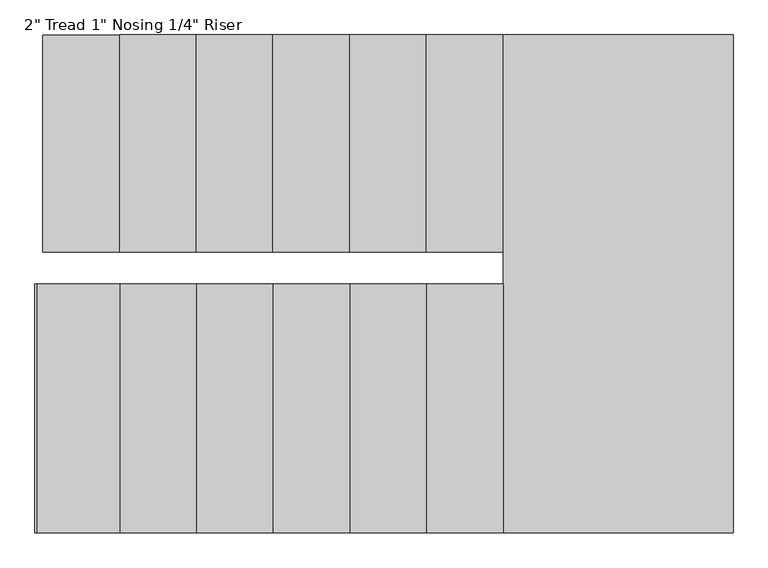
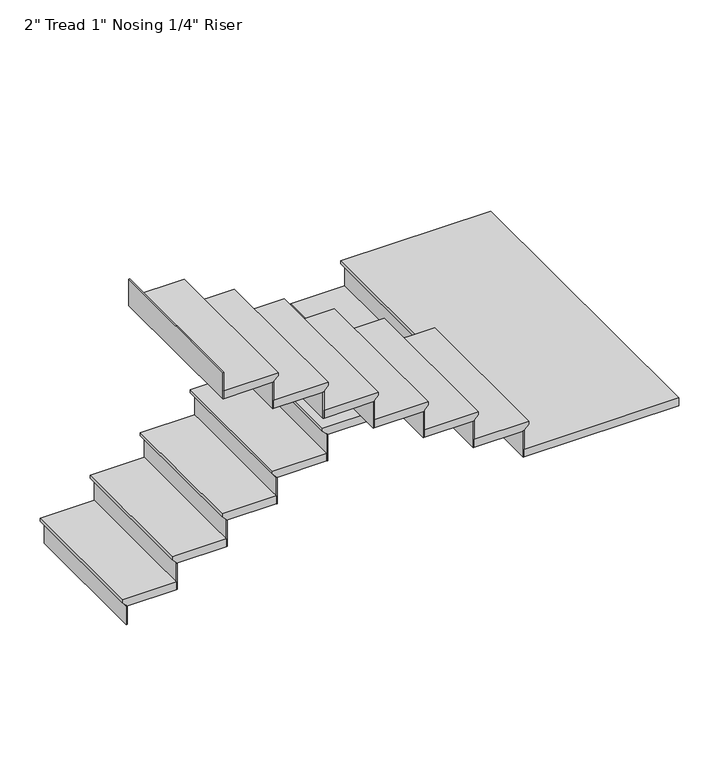
"""IFC4 building model written with IfcOpenShell, lengths in millimetres: stair flight geometry."""

from ifc_helpers import new_model, si_unit, origin, place, context, project, spatial, faceted_brep, source, transform, mapped, element, save


def stair_flight_2c0e0b85(model_context):
    return source(origin(), model_context, "Body", "Brep", [
        faceted_brep([(-879.540747, -2928.9064015, 150.2833333), (-879.540747, -2928.9064015, 169.3333333), (-879.540747, -2065.3064015, 169.3333333), (-879.540747, -2065.3064015, 150.2833333), (-854.140747, -2928.9064015, 124.8833333), (-854.140747, -2065.3064015, 124.8833333), (-549.340747, -2928.9064015, 169.3333333), (-549.340747, -2065.3064015, 169.3333333), (-854.140747, -2065.3064015, 118.5333333), (-549.340747, -2065.3064015, 118.5333333), (-549.340747, -2928.9064015, 118.5333333), (-854.140747, -2928.9064015, 118.5333333)], [[[0, 1, 2, 3]], [[4, 0, 3, 5]], [[2, 1, 6, 7]], [[8, 9, 10, 11]], [[2, 7, 9, 8, 5, 3]], [[8, 11, 4, 5]], [[6, 1, 0, 4, 11, 10]], [[7, 6, 10, 9]]]),
        faceted_brep([(-854.140747, -2928.9064015, 118.5333333), (-854.140747, -2928.9064015, 0.0), (-847.790747, -2928.9064015, 0.0), (-847.790747, -2928.9064015, 118.5333333), (-854.140747, -2065.3064015, 118.5333333), (-847.790747, -2065.3064015, 118.5333333), (-847.790747, -2065.3064015, 0.0), (-854.140747, -2065.3064015, 0.0)], [[[0, 1, 2, 3]], [[4, 5, 6, 7]], [[1, 0, 4, 7]], [[2, 1, 7, 6]], [[3, 2, 6, 5]], [[0, 3, 5, 4]]]),
        faceted_brep([(-549.340747, -2928.9064015, 287.8666667), (-549.340747, -2928.9064015, 118.5333333), (-542.990747, -2928.9064015, 118.5333333), (-542.990747, -2928.9064015, 287.8666667), (-549.340747, -2065.3064015, 287.8666667), (-542.990747, -2065.3064015, 287.8666667), (-542.990747, -2065.3064015, 118.5333333), (-549.340747, -2065.3064015, 118.5333333)], [[[0, 1, 2, 3]], [[4, 5, 6, 7]], [[1, 0, 4, 7]], [[2, 1, 7, 6]], [[3, 2, 6, 5]], [[0, 3, 5, 4]]]),
        faceted_brep([(-574.740747, -2065.3064015, 338.6666667), (-574.740747, -2928.9064015, 338.6666667), (-244.540747, -2928.9064015, 338.6666667), (-244.540747, -2065.3064015, 338.6666667), (-549.340747, -2065.3064015, 287.8666667), (-244.540747, -2065.3064015, 287.8666667), (-244.540747, -2928.9064015, 287.8666667), (-549.340747, -2928.9064015, 287.8666667), (-549.340747, -2065.3064015, 294.2166667), (-574.740747, -2065.3064015, 319.6166667), (-549.340747, -2928.9064015, 294.2166667), (-574.740747, -2928.9064015, 319.6166667)], [[[0, 1, 2, 3]], [[4, 5, 6, 7]], [[0, 3, 5, 4, 8, 9]], [[4, 7, 10, 8]], [[2, 1, 11, 10, 7, 6]], [[3, 2, 6, 5]], [[11, 1, 0, 9]], [[10, 11, 9, 8]]]),
        faceted_brep([(-244.540747, -2928.9064015, 457.2), (-244.540747, -2928.9064015, 287.8666667), (-238.190747, -2928.9064015, 287.8666667), (-238.190747, -2928.9064015, 457.2), (-244.540747, -2065.3064015, 457.2), (-238.190747, -2065.3064015, 457.2), (-238.190747, -2065.3064015, 287.8666667), (-244.540747, -2065.3064015, 287.8666667)], [[[0, 1, 2, 3]], [[4, 5, 6, 7]], [[1, 0, 4, 7]], [[2, 1, 7, 6]], [[3, 2, 6, 5]], [[0, 3, 5, 4]]]),
        faceted_brep([(-269.940747, -2065.3064015, 508.0), (-269.940747, -2928.9064015, 508.0), (60.259253, -2928.9064015, 508.0), (60.259253, -2065.3064015, 508.0), (-244.540747, -2065.3064015, 457.2), (60.259253, -2065.3064015, 457.2), (60.259253, -2928.9064015, 457.2), (-244.540747, -2928.9064015, 457.2), (-244.540747, -2065.3064015, 463.55), (-269.940747, -2065.3064015, 488.95), (-244.540747, -2928.9064015, 463.55), (-269.940747, -2928.9064015, 488.95)], [[[0, 1, 2, 3]], [[4, 5, 6, 7]], [[0, 3, 5, 4, 8, 9]], [[4, 7, 10, 8]], [[2, 1, 11, 10, 7, 6]], [[3, 2, 6, 5]], [[11, 1, 0, 9]], [[10, 11, 9, 8]]]),
        faceted_brep([(60.259253, -2928.9064015, 626.5333333), (60.259253, -2928.9064015, 457.2), (66.609253, -2928.9064015, 457.2), (66.609253, -2928.9064015, 626.5333333), (60.259253, -2065.3064015, 626.5333333), (66.609253, -2065.3064015, 626.5333333), (66.609253, -2065.3064015, 457.2), (60.259253, -2065.3064015, 457.2)], [[[0, 1, 2, 3]], [[4, 5, 6, 7]], [[1, 0, 4, 7]], [[2, 1, 7, 6]], [[3, 2, 6, 5]], [[0, 3, 5, 4]]]),
        faceted_brep([(34.859253, -2065.3064015, 677.3333333), (34.859253, -2928.9064015, 677.3333333), (365.059253, -2928.9064015, 677.3333333), (365.059253, -2065.3064015, 677.3333333), (60.259253, -2065.3064015, 626.5333333), (365.059253, -2065.3064015, 626.5333333), (365.059253, -2928.9064015, 626.5333333), (60.259253, -2928.9064015, 626.5333333), (60.259253, -2065.3064015, 632.8833333), (34.859253, -2065.3064015, 658.2833333), (60.259253, -2928.9064015, 632.8833333), (34.859253, -2928.9064015, 658.2833333)], [[[0, 1, 2, 3]], [[4, 5, 6, 7]], [[0, 3, 5, 4, 8, 9]], [[4, 7, 10, 8]], [[2, 1, 11, 10, 7, 6]], [[3, 2, 6, 5]], [[11, 1, 0, 9]], [[10, 11, 9, 8]]]),
        faceted_brep([(365.059253, -2928.9064015, 795.8666667), (365.059253, -2928.9064015, 626.5333333), (371.409253, -2928.9064015, 626.5333333), (371.409253, -2928.9064015, 795.8666667), (365.059253, -2065.3064015, 795.8666667), (371.409253, -2065.3064015, 795.8666667), (371.409253, -2065.3064015, 626.5333333), (365.059253, -2065.3064015, 626.5333333)], [[[0, 1, 2, 3]], [[4, 5, 6, 7]], [[1, 0, 4, 7]], [[2, 1, 7, 6]], [[3, 2, 6, 5]], [[0, 3, 5, 4]]]),
        faceted_brep([(339.659253, -2065.3064015, 846.6666667), (339.659253, -2928.9064015, 846.6666667), (669.859253, -2928.9064015, 846.6666667), (669.859253, -2065.3064015, 846.6666667), (365.059253, -2065.3064015, 795.8666667), (669.859253, -2065.3064015, 795.8666667), (669.859253, -2928.9064015, 795.8666667), (365.059253, -2928.9064015, 795.8666667), (365.059253, -2065.3064015, 802.2166667), (339.659253, -2065.3064015, 827.6166667), (365.059253, -2928.9064015, 802.2166667), (339.659253, -2928.9064015, 827.6166667)], [[[0, 1, 2, 3]], [[4, 5, 6, 7]], [[0, 3, 5, 4, 8, 9]], [[4, 7, 10, 8]], [[2, 1, 11, 10, 7, 6]], [[3, 2, 6, 5]], [[11, 1, 0, 9]], [[10, 11, 9, 8]]]),
        faceted_brep([(669.859253, -2928.9064015, 965.2), (669.859253, -2928.9064015, 795.8666667), (676.209253, -2928.9064015, 795.8666667), (676.209253, -2928.9064015, 965.2), (669.859253, -2065.3064015, 965.2), (676.209253, -2065.3064015, 965.2), (676.209253, -2065.3064015, 795.8666667), (669.859253, -2065.3064015, 795.8666667)], [[[0, 1, 2, 3]], [[4, 5, 6, 7]], [[1, 0, 4, 7]], [[2, 1, 7, 6]], [[3, 2, 6, 5]], [[0, 3, 5, 4]]]),
        faceted_brep([(644.459253, -2065.3064015, 1016.0), (644.459253, -2928.9064015, 1016.0), (974.659253, -2928.9064015, 1016.0), (974.659253, -2065.3064015, 1016.0), (669.859253, -2065.3064015, 965.2), (974.659253, -2065.3064015, 965.2), (974.659253, -2928.9064015, 965.2), (669.859253, -2928.9064015, 965.2), (669.859253, -2065.3064015, 971.55), (644.459253, -2065.3064015, 996.95), (669.859253, -2928.9064015, 971.55), (644.459253, -2928.9064015, 996.95)], [[[0, 1, 2, 3]], [[4, 5, 6, 7]], [[0, 3, 5, 4, 8, 9]], [[4, 7, 10, 8]], [[2, 1, 11, 10, 7, 6]], [[3, 2, 6, 5]], [[11, 1, 0, 9]], [[10, 11, 9, 8]]]),
        faceted_brep([(974.659253, -2928.9064015, 1134.5333333), (974.659253, -2928.9064015, 965.2), (981.009253, -2928.9064015, 965.2), (981.009253, -2928.9064015, 1134.5333333), (974.659253, -2065.3064015, 1134.5333333), (981.009253, -2065.3064015, 1134.5333333), (981.009253, -2065.3064015, 965.2), (974.659253, -2065.3064015, 965.2)], [[[0, 1, 2, 3]], [[4, 5, 6, 7]], [[1, 0, 4, 7]], [[2, 1, 7, 6]], [[3, 2, 6, 5]], [[0, 3, 5, 4]]]),
        faceted_brep([(923.859253, -4046.5064015, 1185.3333333), (1863.659253, -4046.5064015, 1185.3333333), (1863.659253, -2065.3064015, 1185.3333333), (949.259253, -2065.3064015, 1185.3333333), (949.259253, -3055.9064015, 1185.3333333), (923.859253, -3055.9064015, 1185.3333333), (1863.659253, -4046.5064015, 1134.5333333), (923.859253, -4046.5064015, 1134.5333333), (923.859253, -3055.9064015, 1134.5333333), (949.259253, -3055.9064015, 1134.5333333), (949.259253, -2928.9064015, 1134.5333333), (974.659253, -2928.9064015, 1134.5333333), (974.659253, -2065.3064015, 1134.5333333), (1863.659253, -2065.3064015, 1134.5333333), (974.659253, -2065.3064015, 1140.8833333), (949.259253, -2065.3064015, 1166.2833333), (974.659253, -2928.9064015, 1140.8833333), (949.259253, -2928.9064015, 1166.2833333)], [[[0, 1, 2, 3, 4, 5]], [[6, 7, 8, 9, 10, 11, 12, 13]], [[1, 0, 7, 6]], [[2, 1, 6, 13]], [[3, 2, 13, 12, 14, 15]], [[12, 11, 16, 14]], [[11, 10, 17, 16]], [[4, 3, 15, 17, 10, 9]], [[5, 4, 9, 8]], [[0, 5, 8, 7]], [[15, 14, 16, 17]]]),
        faceted_brep([(923.859253, -3055.9064015, 1303.8666667), (923.859253, -3055.9064015, 1134.5333333), (917.509253, -3055.9064015, 1134.5333333), (917.509253, -3055.9064015, 1303.8666667), (923.859253, -4046.5064015, 1303.8666667), (917.509253, -4046.5064015, 1303.8666667), (917.509253, -4046.5064015, 1134.5333333), (923.859253, -4046.5064015, 1134.5333333)], [[[0, 1, 2, 3]], [[4, 5, 6, 7]], [[1, 0, 4, 7]], [[2, 1, 7, 6]], [[3, 2, 6, 5]], [[0, 3, 5, 4]]]),
        faceted_brep([(949.259253, -4046.5064015, 1354.6666667), (949.259253, -3055.9064015, 1354.6666667), (619.059253, -3055.9064015, 1354.6666667), (619.059253, -4046.5064015, 1354.6666667), (923.859253, -4046.5064015, 1303.8666667), (619.059253, -4046.5064015, 1303.8666667), (619.059253, -3055.9064015, 1303.8666667), (923.859253, -3055.9064015, 1303.8666667), (923.859253, -4046.5064015, 1310.2166667), (949.259253, -4046.5064015, 1335.6166667), (923.859253, -3055.9064015, 1310.2166667), (949.259253, -3055.9064015, 1335.6166667)], [[[0, 1, 2, 3]], [[4, 5, 6, 7]], [[0, 3, 5, 4, 8, 9]], [[4, 7, 10, 8]], [[2, 1, 11, 10, 7, 6]], [[3, 2, 6, 5]], [[11, 1, 0, 9]], [[10, 11, 9, 8]]]),
        faceted_brep([(619.059253, -3055.9064015, 1473.2), (619.059253, -3055.9064015, 1303.8666667), (612.709253, -3055.9064015, 1303.8666667), (612.709253, -3055.9064015, 1473.2), (619.059253, -4046.5064015, 1473.2), (612.709253, -4046.5064015, 1473.2), (612.709253, -4046.5064015, 1303.8666667), (619.059253, -4046.5064015, 1303.8666667)], [[[0, 1, 2, 3]], [[4, 5, 6, 7]], [[1, 0, 4, 7]], [[2, 1, 7, 6]], [[3, 2, 6, 5]], [[0, 3, 5, 4]]]),
        faceted_brep([(644.459253, -4046.5064015, 1524.0), (644.459253, -3055.9064015, 1524.0), (314.259253, -3055.9064015, 1524.0), (314.259253, -4046.5064015, 1524.0), (619.059253, -4046.5064015, 1473.2), (314.259253, -4046.5064015, 1473.2), (314.259253, -3055.9064015, 1473.2), (619.059253, -3055.9064015, 1473.2), (619.059253, -4046.5064015, 1479.55), (644.459253, -4046.5064015, 1504.95), (619.059253, -3055.9064015, 1479.55), (644.459253, -3055.9064015, 1504.95)], [[[0, 1, 2, 3]], [[4, 5, 6, 7]], [[0, 3, 5, 4, 8, 9]], [[4, 7, 10, 8]], [[2, 1, 11, 10, 7, 6]], [[3, 2, 6, 5]], [[11, 1, 0, 9]], [[10, 11, 9, 8]]]),
        faceted_brep([(314.259253, -3055.9064015, 1642.5333333), (314.259253, -3055.9064015, 1473.2), (307.909253, -3055.9064015, 1473.2), (307.909253, -3055.9064015, 1642.5333333), (314.259253, -4046.5064015, 1642.5333333), (307.909253, -4046.5064015, 1642.5333333), (307.909253, -4046.5064015, 1473.2), (314.259253, -4046.5064015, 1473.2)], [[[0, 1, 2, 3]], [[4, 5, 6, 7]], [[1, 0, 4, 7]], [[2, 1, 7, 6]], [[3, 2, 6, 5]], [[0, 3, 5, 4]]]),
        faceted_brep([(339.659253, -4046.5064015, 1693.3333333), (339.659253, -3055.9064015, 1693.3333333), (9.459253, -3055.9064015, 1693.3333333), (9.459253, -4046.5064015, 1693.3333333), (314.259253, -4046.5064015, 1642.5333333), (9.459253, -4046.5064015, 1642.5333333), (9.459253, -3055.9064015, 1642.5333333), (314.259253, -3055.9064015, 1642.5333333), (314.259253, -4046.5064015, 1648.8833333), (339.659253, -4046.5064015, 1674.2833333), (314.259253, -3055.9064015, 1648.8833333), (339.659253, -3055.9064015, 1674.2833333)], [[[0, 1, 2, 3]], [[4, 5, 6, 7]], [[0, 3, 5, 4, 8, 9]], [[4, 7, 10, 8]], [[2, 1, 11, 10, 7, 6]], [[3, 2, 6, 5]], [[11, 1, 0, 9]], [[10, 11, 9, 8]]]),
        faceted_brep([(9.459253, -3055.9064015, 1811.8666667), (9.459253, -3055.9064015, 1642.5333333), (3.109253, -3055.9064015, 1642.5333333), (3.109253, -3055.9064015, 1811.8666667), (9.459253, -4046.5064015, 1811.8666667), (3.109253, -4046.5064015, 1811.8666667), (3.109253, -4046.5064015, 1642.5333333), (9.459253, -4046.5064015, 1642.5333333)], [[[0, 1, 2, 3]], [[4, 5, 6, 7]], [[1, 0, 4, 7]], [[2, 1, 7, 6]], [[3, 2, 6, 5]], [[0, 3, 5, 4]]]),
        faceted_brep([(34.859253, -4046.5064015, 1862.6666667), (34.859253, -3055.9064015, 1862.6666667), (-295.340747, -3055.9064015, 1862.6666667), (-295.340747, -4046.5064015, 1862.6666667), (9.459253, -4046.5064015, 1811.8666667), (-295.340747, -4046.5064015, 1811.8666667), (-295.340747, -3055.9064015, 1811.8666667), (9.459253, -3055.9064015, 1811.8666667), (9.459253, -4046.5064015, 1818.2166667), (34.859253, -4046.5064015, 1843.6166667), (9.459253, -3055.9064015, 1818.2166667), (34.859253, -3055.9064015, 1843.6166667)], [[[0, 1, 2, 3]], [[4, 5, 6, 7]], [[0, 3, 5, 4, 8, 9]], [[4, 7, 10, 8]], [[2, 1, 11, 10, 7, 6]], [[3, 2, 6, 5]], [[11, 1, 0, 9]], [[10, 11, 9, 8]]]),
        faceted_brep([(-295.340747, -3055.9064015, 1981.2), (-295.340747, -3055.9064015, 1811.8666667), (-301.690747, -3055.9064015, 1811.8666667), (-301.690747, -3055.9064015, 1981.2), (-295.340747, -4046.5064015, 1981.2), (-301.690747, -4046.5064015, 1981.2), (-301.690747, -4046.5064015, 1811.8666667), (-295.340747, -4046.5064015, 1811.8666667)], [[[0, 1, 2, 3]], [[4, 5, 6, 7]], [[1, 0, 4, 7]], [[2, 1, 7, 6]], [[3, 2, 6, 5]], [[0, 3, 5, 4]]]),
        faceted_brep([(-269.940747, -4046.5064015, 2032.0), (-269.940747, -3055.9064015, 2032.0), (-600.140747, -3055.9064015, 2032.0), (-600.140747, -4046.5064015, 2032.0), (-295.340747, -4046.5064015, 1981.2), (-600.140747, -4046.5064015, 1981.2), (-600.140747, -3055.9064015, 1981.2), (-295.340747, -3055.9064015, 1981.2), (-295.340747, -4046.5064015, 1987.55), (-269.940747, -4046.5064015, 2012.95), (-295.340747, -3055.9064015, 1987.55), (-269.940747, -3055.9064015, 2012.95)], [[[0, 1, 2, 3]], [[4, 5, 6, 7]], [[0, 3, 5, 4, 8, 9]], [[4, 7, 10, 8]], [[2, 1, 11, 10, 7, 6]], [[3, 2, 6, 5]], [[11, 1, 0, 9]], [[10, 11, 9, 8]]]),
        faceted_brep([(-600.140747, -3055.9064015, 2150.5333333), (-600.140747, -3055.9064015, 1981.2), (-606.490747, -3055.9064015, 1981.2), (-606.490747, -3055.9064015, 2150.5333333), (-600.140747, -4046.5064015, 2150.5333333), (-606.490747, -4046.5064015, 2150.5333333), (-606.490747, -4046.5064015, 1981.2), (-600.140747, -4046.5064015, 1981.2)], [[[0, 1, 2, 3]], [[4, 5, 6, 7]], [[1, 0, 4, 7]], [[2, 1, 7, 6]], [[3, 2, 6, 5]], [[0, 3, 5, 4]]]),
        faceted_brep([(-904.940747, -3055.9064015, 2319.8666667), (-904.940747, -3055.9064015, 2150.5333333), (-911.290747, -3055.9064015, 2150.5333333), (-911.290747, -3055.9064015, 2319.8666667), (-904.940747, -4046.5064015, 2319.8666667), (-911.290747, -4046.5064015, 2319.8666667), (-911.290747, -4046.5064015, 2150.5333333), (-904.940747, -4046.5064015, 2150.5333333)], [[[0, 1, 2, 3]], [[4, 5, 6, 7]], [[1, 0, 4, 7]], [[2, 1, 7, 6]], [[3, 2, 6, 5]], [[0, 3, 5, 4]]]),
        faceted_brep([(-574.740747, -4046.5064015, 2201.3333333), (-574.740747, -3055.9064015, 2201.3333333), (-904.940747, -3055.9064015, 2201.3333333), (-904.940747, -4046.5064015, 2201.3333333), (-600.140747, -4046.5064015, 2150.5333333), (-904.940747, -4046.5064015, 2150.5333333), (-904.940747, -3055.9064015, 2150.5333333), (-600.140747, -3055.9064015, 2150.5333333), (-600.140747, -4046.5064015, 2156.8833333), (-574.740747, -4046.5064015, 2182.2833333), (-600.140747, -3055.9064015, 2156.8833333), (-574.740747, -3055.9064015, 2182.2833333)], [[[0, 1, 2, 3]], [[4, 5, 6, 7]], [[0, 3, 5, 4, 8, 9]], [[4, 7, 10, 8]], [[2, 1, 11, 10, 7, 6]], [[3, 2, 6, 5]], [[11, 1, 0, 9]], [[10, 11, 9, 8]]]),
    ])


if __name__ == "__main__":
    model = new_model("IFC4")
    model_context = context("Model", 3, world=origin())
    ifc_project = project(units=[si_unit("LENGTHUNIT", "METRE", prefix="MILLI")], contexts=[model_context])
    site = spatial("IfcSite", under=ifc_project)
    building = spatial("IfcBuilding", under=site)
    placement = place(None, origin())
    stair_flight_shape = stair_flight_2c0e0b85(model_context)
    element("IfcStairFlight", 1, ObjectType="2\" Tread 1\" Nosing 1/4\" Riser", at=placement, inside=building, context=model_context, shape_type="MappedRepresentation", body=[
        mapped(stair_flight_shape, transform((0.0, 0.0, 0.0), x_axis=(1.0, 0.0, 0.0), y_axis=(0.0, 1.0, 0.0), z_axis=(0.0, 0.0, 1.0))),
    ])
    save(model, "model.ifc")
